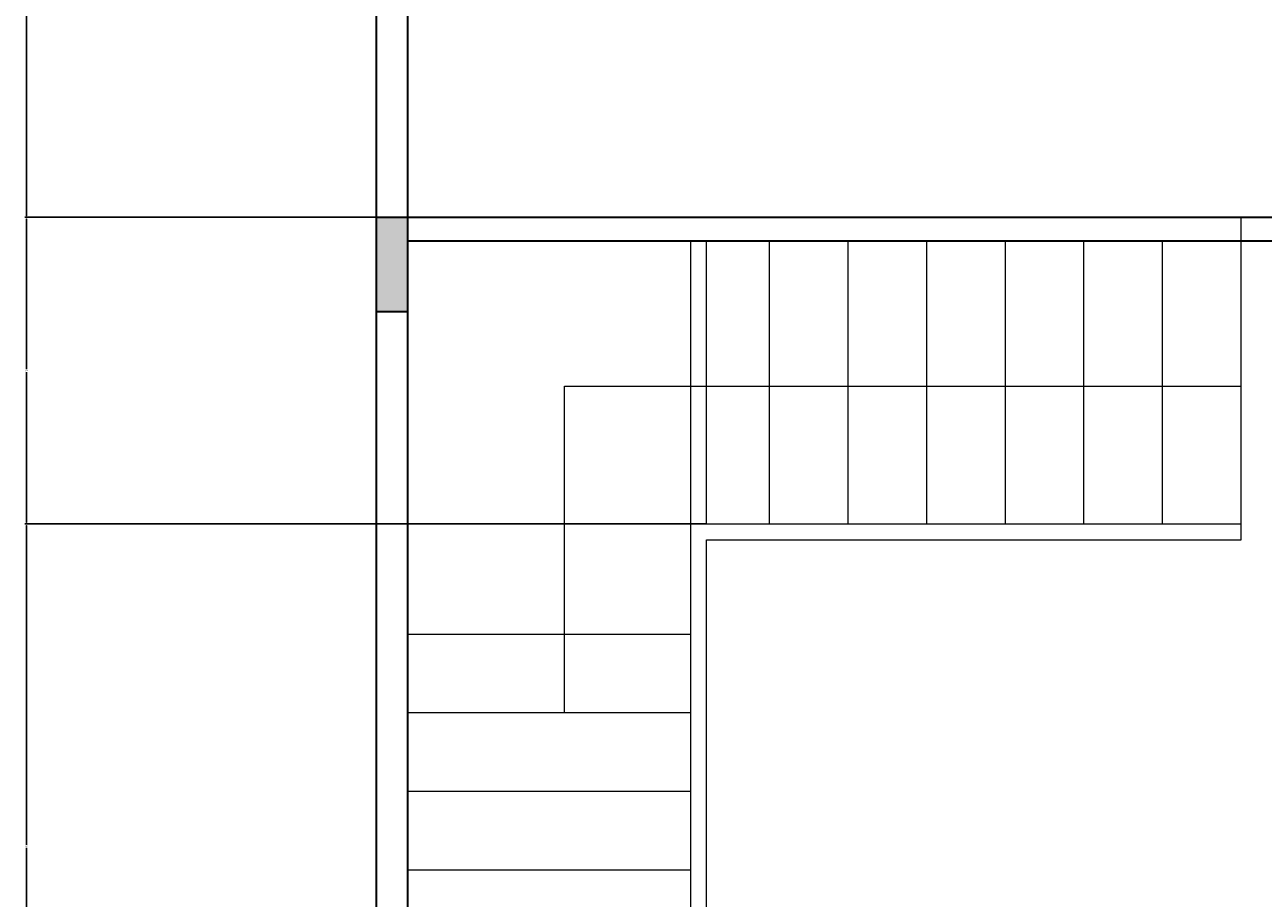
# Model space of a CAD drawing. Units: inches. Extents: x 1002 to 1561, y 1016 to 1994.
# Tile 5 of 8: x 1002 to 1159, y 1394 to 1505. Entities that reach past the tile are written whole.
import ezdxf

# ---------------------------------------------------------------- set-up
doc = ezdxf.new("R2010")
doc.units = ezdxf.units.IN
doc.header["$MEASUREMENT"] = 0
for name, color, linetype, lineweight in [('A-ANNO-DIMS', 2, 'Continuous', 18), ('A-WALL', 7, 'Continuous', 35), ('A-WALL-PATT', 7, 'Continuous', 13)]:
    doc.layers.add(name, color=color, linetype=linetype, lineweight=lineweight)
doc.layers.add('A-FLOR-STRS', color=217, linetype='Continuous', lineweight=18, true_color=0x93278f)
doc.styles.get("Standard").update_dxf_attribs({"font": 'arial.ttf'})
doc.dimstyles.get("Standard").update_dxf_attribs({"dimtxt": 0.18, "dimasz": 0.18, "dimexe": 0.18, "dimexo": 0.0625, "dimgap": 0.09, "dimtad": 0, "dimtih": 1, "dimtoh": 1, "dimdec": 4, "dimzin": 0, "dimdsep": 46, "dimtxsty": 'Standard', "dimcen": 0.09, "dimadec": 0, "dimazin": 0, "dimtfac": 1, "dimtdec": 4, "dimtofl": 0, "dimtmove": 0, "dimatfit": 3, "dimfxl": 1, "dimtolj": 1, "dimtzin": 0, "dimarcsym": 0})

# ---------------------------------------------------------------- blocks, each defined once
blk = doc.blocks.new('*D11')
at = {"layer": 'A-ANNO-DIMS', "color": 0, "lineweight": -2, "transparency": 16777216}
for p, q in [((1046.37, 1645.51), (1001.74, 1645.51)), ((1001.92, 1645.33), (1001.92, 1563.19)), ((1001.92, 1480.69), (1001.92, 1562.83)), ((1046.37, 1480.51), (1001.74, 1480.51))]:
    blk.add_line(p, q, dxfattribs=at)
at = {"layer": 'A-ANNO-DIMS', "color": 0, "transparency": 16777216}
for points in [[(1001.89, 1645.33), (1001.95, 1645.33), (1001.92, 1645.51)], [(1001.89, 1480.69), (1001.95, 1480.69), (1001.92, 1480.51)]]:
    blk.add_solid(points, dxfattribs=at)
at = {"layer": 'Defpoints', "color": 0, "transparency": 16777216}
for p in [(1001.92, 1645.51), (1046.43, 1645.51), (1046.43, 1480.51)]:
    blk.add_point(p, dxfattribs=at)
at = {"layer": 'A-ANNO-DIMS', "color": 0, "transparency": 16777216, "insert": (1001.92, 1563.01), "char_height": 0.18, "attachment_point": 5}
blk.add_mtext('\\A1;165', dxfattribs=at)
blk = doc.blocks.new('*D12')
at = {"layer": 'A-ANNO-DIMS', "color": 0, "lineweight": -2, "transparency": 16777216}
for p, q in [((1046.37, 1480.51), (1001.74, 1480.51)), ((1001.92, 1480.33), (1001.92, 1461.19)), ((1001.92, 1441.69), (1001.92, 1460.83)), ((1088.37, 1441.51), (1001.74, 1441.51))]:
    blk.add_line(p, q, dxfattribs=at)
at = {"layer": 'A-ANNO-DIMS', "color": 0, "transparency": 16777216}
for points in [[(1001.89, 1480.33), (1001.95, 1480.33), (1001.92, 1480.51)], [(1001.89, 1441.69), (1001.95, 1441.69), (1001.92, 1441.51)]]:
    blk.add_solid(points, dxfattribs=at)
at = {"layer": 'Defpoints', "color": 0, "transparency": 16777216}
for p in [(1001.92, 1480.51), (1046.43, 1480.51), (1088.43, 1441.51)]:
    blk.add_point(p, dxfattribs=at)
at = {"layer": 'A-ANNO-DIMS', "color": 0, "transparency": 16777216, "insert": (1001.92, 1461.01), "char_height": 0.18, "attachment_point": 5}
blk.add_mtext('\\A1;39', dxfattribs=at)
blk = doc.blocks.new('*D13')
at = {"layer": 'A-ANNO-DIMS', "color": 0, "lineweight": -2, "transparency": 16777216}
for p, q in [((1088.37, 1441.51), (1001.74, 1441.51)), ((1001.92, 1441.33), (1001.92, 1400.69)), ((1001.92, 1359.69), (1001.92, 1400.33)), ((1086.37, 1359.51), (1001.74, 1359.51))]:
    blk.add_line(p, q, dxfattribs=at)
at = {"layer": 'A-ANNO-DIMS', "color": 0, "transparency": 16777216}
for points in [[(1001.89, 1441.33), (1001.95, 1441.33), (1001.92, 1441.51)], [(1001.89, 1359.69), (1001.95, 1359.69), (1001.92, 1359.51)]]:
    blk.add_solid(points, dxfattribs=at)
at = {"layer": 'Defpoints', "color": 0, "transparency": 16777216}
for p in [(1001.92, 1441.51), (1088.43, 1441.51), (1086.43, 1359.51)]:
    blk.add_point(p, dxfattribs=at)
at = {"layer": 'A-ANNO-DIMS', "color": 0, "transparency": 16777216, "insert": (1001.92, 1400.51), "char_height": 0.18, "attachment_point": 5}
blk.add_mtext('\\A1;82', dxfattribs=at)

msp = doc.modelspace()

# ---------------------------------------------------------------- hatches: boundary and pattern name
at = {"layer": 'A-WALL-PATT'}
h = msp.add_hatch(color=256, dxfattribs=at)
h.dxf.hatch_style = 1
h.paths.add_polyline_path([(1206.434, 1924.784), (1203.434, 1924.784), (1203.434, 1898.155), (1206.434, 1898.155)])
h.paths.add_polyline_path([(1326.434, 1925.745), (1323.434, 1925.745), (1323.434, 1900.458), (1326.434, 1900.458)])
h.paths.add_polyline_path([(1290.434, 1840.51), (1287.434, 1840.51), (1287.434, 1837.51), (1287.434, 1823.284), (1290.434, 1823.284)])
h.paths.add_polyline_path([(1287.434, 1840.51), (1285.684, 1840.51), (1285.684, 1837.51), (1287.434, 1837.51)])
h.paths.add_polyline_path([(1233.434, 1840.51), (1230.434, 1840.51), (1230.434, 1823.284), (1233.434, 1823.284)])
h.paths.add_polyline_path([(1235.119, 1840.51), (1233.434, 1840.51), (1233.434, 1837.51), (1235.119, 1837.51)])
h.paths.add_polyline_path([(1050.434, 1837.51), (1050.434, 1840.51), (1046.434, 1840.51), (1046.434, 1814.619), (1050.434, 1814.619)])
h.paths.add_polyline_path([(1050.434, 1682.088), (1046.434, 1682.088), (1046.434, 1648.51), (1046.434, 1645.51), (1050.434, 1645.51), (1050.434, 1648.51)])
h.paths.add_polyline_path([(1233.434, 1648.51), (1211.636, 1648.51), (1211.636, 1645.51), (1233.434, 1645.51)])
h.paths.add_polyline_path([(1307.549, 1648.51), (1287.434, 1648.51), (1287.434, 1645.51), (1307.549, 1645.51)])
h.paths.add_polyline_path([(1516.434, 1927.595), (1512.434, 1927.595), (1512.434, 1896.846), (1516.434, 1896.846)])
h.paths.add_polyline_path([(1516.434, 1840.51), (1512.434, 1840.51), (1512.434, 1816.31), (1516.434, 1816.31)])
h.paths.add_polyline_path([(1516.434, 1686.827), (1512.434, 1686.827), (1512.434, 1645.51), (1516.434, 1645.51)])
h.paths.add_polyline_path([(1472.434, 1321.51), (1469.434, 1321.51), (1469.434, 1306.51), (1472.434, 1306.51)])
h.paths.add_polyline_path([(1295.733, 1141.51), (1281.793, 1141.51), (1281.793, 1137.51), (1295.733, 1137.51)])
h.paths.add_polyline_path([(1239.434, 1321.51), (1230.434, 1321.51), (1230.434, 1318.51), (1239.434, 1318.51)])
h.paths.add_polyline_path([(1290.434, 1332.122), (1287.434, 1332.122), (1287.434, 1318.51), (1290.434, 1318.51)])
h.paths.add_polyline_path([(1311.434, 1480.51), (1287.434, 1480.51), (1287.434, 1477.51), (1311.434, 1477.51)])
h.paths.add_polyline_path([(1050.434, 1480.51), (1046.434, 1480.51), (1046.434, 1468.51), (1050.434, 1468.51)])
h.paths.add_polyline_path([(1050.434, 1321.51), (1046.434, 1321.51), (1046.434, 1309.51), (1050.434, 1309.51)])
h.paths.add_polyline_path([(1233.434, 1192.382), (1230.434, 1192.382), (1230.434, 1168.702), (1233.434, 1168.702)])
h.paths.add_polyline_path([(1050.434, 1137.51), (1046.434, 1137.51), (1046.434, 1119.51), (1050.434, 1119.51)])
h.paths.add_polyline_path([(1472.434, 1153.51), (1469.434, 1153.51), (1469.434, 1141.51), (1472.434, 1141.51)])
h.paths.add_polyline_path([(1472.434, 1141.51), (1469.434, 1141.51), (1469.434, 1137.51), (1472.434, 1137.51)])

# ---------------------------------------------------------------- linework, layer by layer
at = {"layer": 'A-FLOR-STRS'}
for p, q in [((1156.434, 1439.51), (1156.434, 1480.51)), ((1086.434, 1417.51), (1086.434, 1477.51)), ((1086.434, 1417.51), (1086.434, 1477.51)), ((1088.434, 1441.51), (1088.434, 1477.51)), ((1096.434, 1441.51), (1096.434, 1477.51)), ((1106.434, 1441.51), (1106.434, 1477.51)), ((1116.434, 1441.51), (1116.434, 1477.51)), ((1126.434, 1441.51), (1126.434, 1477.51)), ((1136.434, 1441.51), (1136.434, 1477.51)), ((1146.434, 1441.51), (1146.434, 1477.51)), ((1070.363, 1459.046), (1156.434, 1459.046)), ((1070.363, 1417.51), (1070.363, 1459.046)), ((1050.434, 1441.51), (1156.434, 1441.51)), ((1088.434, 1439.51), (1156.434, 1439.51)), ((1088.434, 1417.51), (1088.434, 1439.51)), ((1050.434, 1427.51), (1086.434, 1427.51)), ((1050.434, 1417.51), (1086.434, 1417.51)), ((1086.434, 1321.51), (1086.434, 1417.51)), ((1088.434, 1359.51), (1088.434, 1417.51)), ((1050.434, 1407.51), (1086.434, 1407.51)), ((1050.434, 1397.51), (1086.434, 1397.51))]:
    msp.add_line(p, q, dxfattribs=at)
at = {"layer": 'A-WALL'}
for p, q in [((1046.434, 1119.51), (1046.434, 1682.088)), ((1050.434, 1119.51), (1050.434, 1682.088)), ((1046.434, 1480.51), (1156.434, 1480.51)), ((1156.434, 1480.51), (1213.471, 1480.51)), ((1050.434, 1477.51), (1156.434, 1477.51)), ((1156.434, 1477.51), (1213.471, 1477.51)), ((1046.434, 1468.51), (1050.434, 1468.51))]:
    msp.add_line(p, q, dxfattribs=at)

# ---------------------------------------------------------------- dimensions: what is measured, and where the dimension line sits
at = {"layer": 'A-ANNO-DIMS'}
for base, p1, p2, picture, middle in [((1001.924, 1645.51), (1046.434, 1480.51), (1046.434, 1645.51), '*D11', (1001.924, 1563.01)), ((1001.924, 1480.51), (1088.434, 1441.51), (1046.434, 1480.51), '*D12', (1001.924, 1461.01)), ((1001.924, 1441.51), (1086.434, 1359.51), (1088.434, 1441.51), '*D13', (1001.924, 1400.51))]:
    dim = msp.add_linear_dim(base=base, p1=p1, p2=p2, angle=90, dimstyle='Standard', override={"dimdec": 0, "dimlfac": 1, "dimrnd": 0, "dimzin": 0, "dimdsep": 46, "dimlunit": 2}, dxfattribs=at)
    dim.commit()
    dim.dimension.update_dxf_attribs({"geometry": picture, "text_midpoint": middle})

doc.saveas('drawing.dxf')
